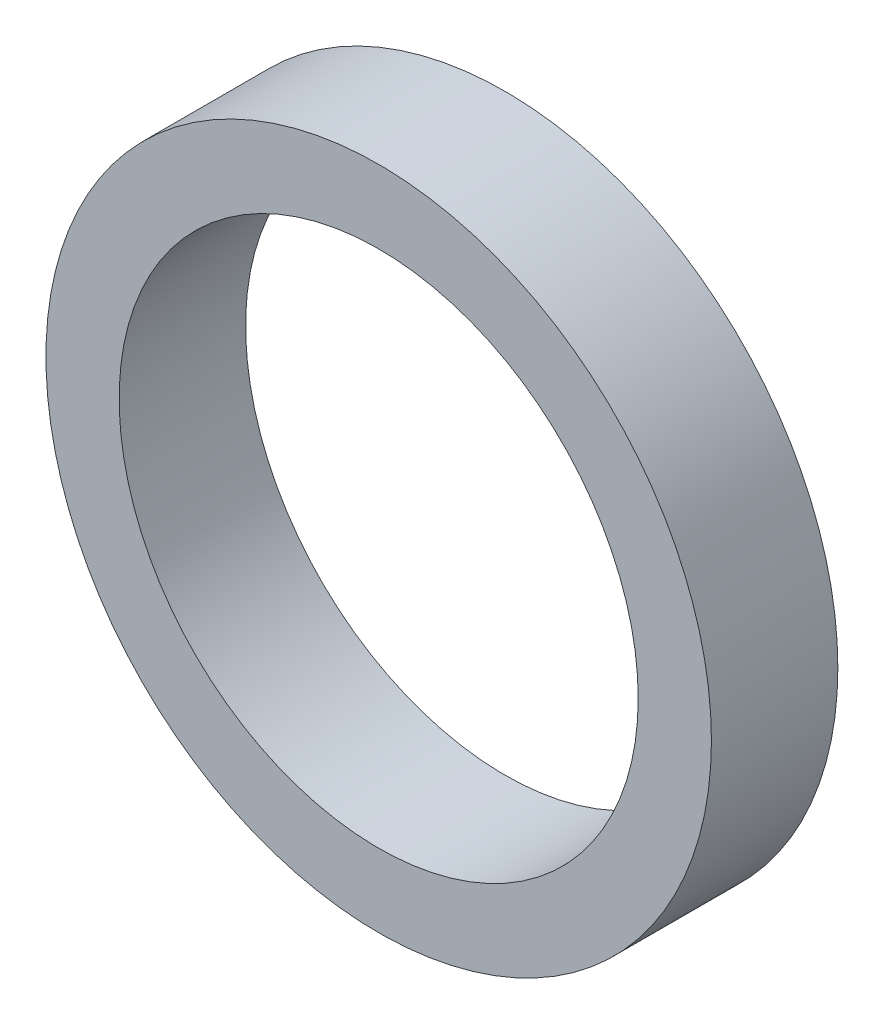
from build123d import *

# Parameters (mm, degrees)
BUSH_RING_PROFILE_0_500_X_0_390_R   = 6.35
BUSH_RING_PROFILE_0_500_X_0_390_R_2 = 4.953
BUSH_RING_0_095_THICK_DEPTH         = 2.413


with BuildPart() as part:
    # Bush Ring Profile Ø0.500 x Ø0.390 → Bush Ring 0.095 Thick (new body)
    with BuildSketch(Plane.XY):
        Circle(BUSH_RING_PROFILE_0_500_X_0_390_R)
        Circle(BUSH_RING_PROFILE_0_500_X_0_390_R_2, mode=Mode.SUBTRACT)
    extrude(amount=BUSH_RING_0_095_THICK_DEPTH)


solid = part.part
